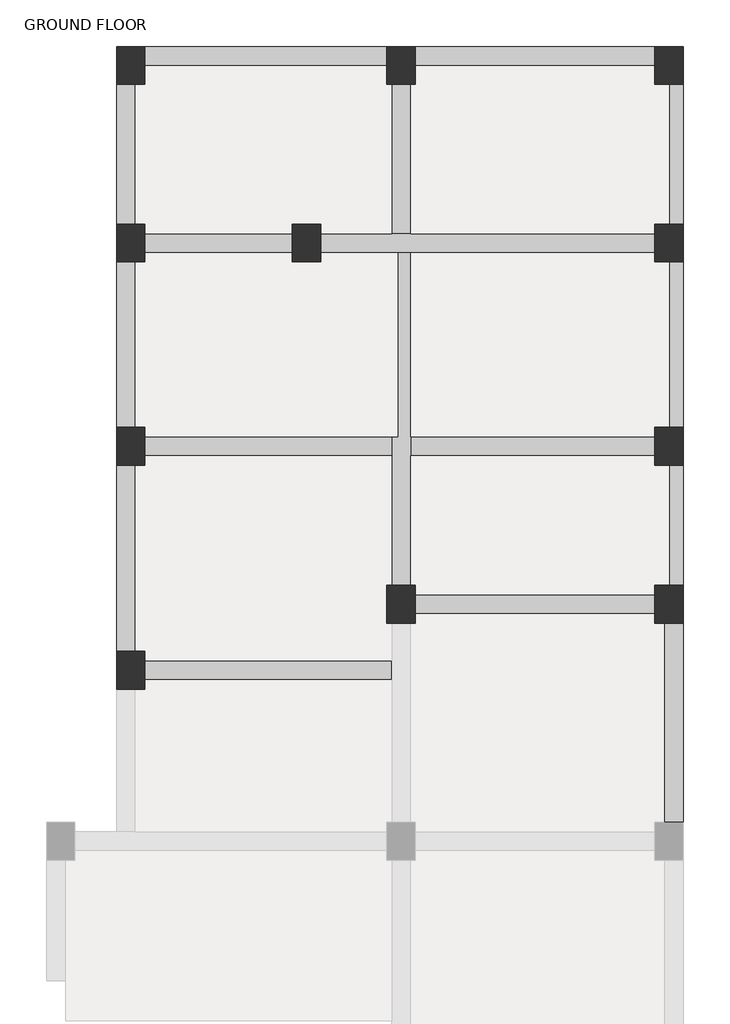
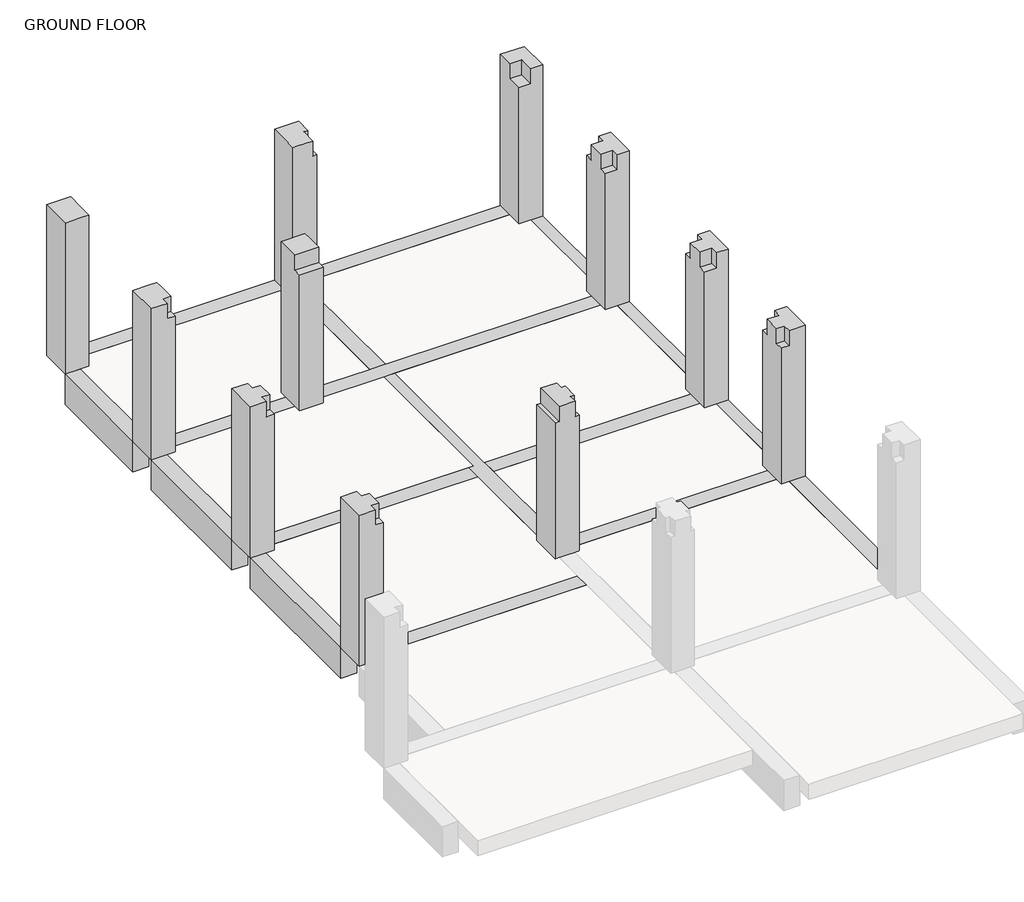
# One storey, part 2 of 2: 17 beams, 11 columns.
"""IFC4 building model written with IfcOpenShell, lengths in millimetres."""

from ifc_helpers import new_model, si_unit, frame, origin, place, context, project, spatial, polyline, outline, extrude, faceted_brep, element, save

model = new_model("IFC4")

# Units and contexts
model_context = context("Model", 3, world=origin())
ifc_project = project(units=[si_unit("LENGTHUNIT", "METRE", prefix="MILLI")], contexts=[model_context])

# Site, building, storey
site = spatial("IfcSite", under=ifc_project)
building = spatial("IfcBuilding", under=site)
storey = spatial("IfcBuildingStorey", under=building, Name="GROUND FLOOR", Elevation=0.0)

# Beams
placement = place(None, origin())
element("IfcBeam", 1, ObjectType="M_Concrete-Rectangular Beam : 300 x 600mm", at=placement, inside=storey, context=model_context, shape_type="Brep", body=[
    faceted_brep([(-2096.635935, 10150.0657956, 0.0), (-2096.635935, 10450.0657956, 0.0), (-5925.9642664, 10450.0657956, 0.0), (-5925.9642664, 10150.0657956, 0.0), (-2096.635935, 10150.0657956, -600.0), (-2096.635935, 10150.0657956, -300.0), (-5925.9642664, 10150.0657956, -300.0), (-5925.9642664, 10150.0657956, -600.0), (-2096.635935, 10450.0657956, -600.0), (-5925.9642664, 10450.0657956, -600.0)], [[[0, 1, 2, 3]], [[4, 5, 0, 3, 6, 7]], [[8, 4, 7, 9]], [[1, 8, 9, 2]], [[2, 9, 7, 6, 3]], [[1, 0, 5, 4, 8]]]),
])
element("IfcBeam", 2, ObjectType="M_Concrete-Rectangular Beam : 300 x 600mm", at=placement, inside=storey, context=model_context, shape_type="SweptSolid", body=[
    extrude(outline(polyline([(2143.5134108, 10450.0657956), (2143.5134108, 10150.0657956), (-1646.635935, 10150.0657956), (-1646.635935, 10450.0657956), (2143.5134108, 10450.0657956)])), frame((0.0, 0.0, -600.0), z_axis=(0.0, 0.0, 1.0), x_axis=(1.0, 0.0, 0.0)), (0.0, 0.0, 1.0), 600.0),
])
element("IfcBeam", 3, ObjectType="M_Concrete-Rectangular Beam : 300 x 600mm", at=placement, inside=storey, context=model_context, shape_type="Brep", body=[
    faceted_brep([(-6375.9642664, 7641.506653, 0.0), (-6075.9642664, 7641.506653, 0.0), (-6075.9642664, 9850.0657956, 0.0), (-6375.9642664, 9850.0657956, 0.0), (-6375.9642664, 7641.506653, -600.0), (-6375.9642664, 9850.0657956, -600.0), (-6075.9642664, 7641.506653, -600.0), (-6075.9642664, 9850.0657956, -600.0), (-6075.9642664, 7641.506653, -300.0), (-6075.9642664, 9850.0657956, -300.0)], [[[0, 1, 2, 3]], [[4, 0, 3, 5]], [[6, 4, 5, 7]], [[1, 8, 6, 7, 9, 2]], [[2, 9, 7, 5, 3]], [[1, 0, 4, 6, 8]]]),
])
element("IfcBeam", 4, ObjectType="M_Concrete-Rectangular Beam : 300 x 600mm", at=placement, inside=storey, context=model_context, shape_type="SweptSolid", body=[
    extrude(outline(polyline([(-6075.9642664, 4424.5351605), (-6375.9642664, 4424.5351605), (-6375.9642664, 7041.506653), (-6075.9642664, 7041.506653), (-6075.9642664, 4424.5351605)])), frame((0.0, 0.0, -600.0), z_axis=(0.0, 0.0, 1.0), x_axis=(1.0, 0.0, 0.0)), (0.0, 0.0, 1.0), 600.0),
])
element("IfcBeam", 5, ObjectType="M_Concrete-Rectangular Beam : 300 x 600mm", at=placement, inside=storey, context=model_context, shape_type="SweptSolid", body=[
    extrude(outline(polyline([(-6075.9642664, 881.5941646), (-6375.9642664, 881.5941646), (-6375.9642664, 3824.5351605), (-6075.9642664, 3824.5351605), (-6075.9642664, 881.5941646)])), frame((0.0, 0.0, -600.0), z_axis=(0.0, 0.0, 1.0), x_axis=(1.0, 0.0, 0.0)), (0.0, 0.0, 1.0), 600.0),
])
element("IfcBeam", 6, ObjectType="M_Concrete-Rectangular Beam : 300 x 600mm", at=placement, inside=storey, context=model_context, shape_type="SweptSolid", body=[
    extrude(outline(polyline([(2293.5134108, 1328.1057379), (2593.5134108, 1328.1057379), (2593.5134108, -1823.3693625), (2293.5134108, -1823.3693625), (2293.5134108, 1328.1057379)])), frame((0.0, 0.0, -600.0), z_axis=(0.0, 0.0, 1.0), x_axis=(1.0, 0.0, 0.0)), (0.0, 0.0, 1.0), 600.0),
])
element("IfcBeam", 7, ObjectType="M_Concrete-Rectangular Beam : 300 x 600mm", at=placement, inside=storey, context=model_context, shape_type="SweptSolid", body=[
    extrude(outline(polyline([(-600.0, 2293.5134108), (-600.0, 2593.5134108), (0.0, 2593.5134108), (0.0, 2368.5134108), (-300.0, 2368.5134108), (-300.0, 2293.5134108), (-600.0, 2293.5134108)])), frame((0.0, 1928.1057379, 0.0), z_axis=(0.0, 1.0, 0.0), x_axis=(0.0, 0.0, 1.0)), (0.0, 0.0, 1.0), 1896.4294226),
])
element("IfcBeam", 8, ObjectType="M_Concrete-Rectangular Beam : 300 x 600mm", at=placement, inside=storey, context=model_context, shape_type="SweptSolid", body=[
    extrude(outline(polyline([(-600.0, 2293.5134108), (-600.0, 2593.5134108), (0.0, 2593.5134108), (0.0, 2368.5134108), (-300.0, 2368.5134108), (-300.0, 2293.5134108), (-600.0, 2293.5134108)])), frame((0.0, 4424.5351605, 0.0), z_axis=(0.0, 1.0, 0.0), x_axis=(0.0, 0.0, 1.0)), (0.0, 0.0, 1.0), 2616.9714925),
])
element("IfcBeam", 9, ObjectType="M_Concrete-Rectangular Beam : 300 x 600mm", at=placement, inside=storey, context=model_context, shape_type="SweptSolid", body=[
    extrude(outline(polyline([(-600.0, 2293.5134108), (-600.0, 2593.5134108), (0.0, 2593.5134108), (0.0, 2368.5134108), (-300.0, 2368.5134108), (-300.0, 2293.5134108), (-600.0, 2293.5134108)])), frame((0.0, 7641.506653, 0.0), z_axis=(0.0, 1.0, 0.0), x_axis=(0.0, 0.0, 1.0)), (0.0, 0.0, 1.0), 2208.5591426),
])
element("IfcBeam", 10, ObjectType="M_Concrete-Rectangular Beam : 300 x 600mm", at=placement, inside=storey, context=model_context, shape_type="Brep", body=[
    faceted_brep([(-3596.635935, 7191.506653, 0.0), (-3596.635935, 7491.506653, 0.0), (-5925.9642664, 7491.506653, 0.0), (-5925.9642664, 7191.506653, 0.0), (-3596.635935, 7191.506653, -600.0), (-5925.9642664, 7191.506653, -600.0), (-3596.635935, 7491.506653, -600.0), (-5925.9642664, 7491.506653, -600.0), (-3596.635935, 7491.506653, -300.0), (-5925.9642664, 7491.506653, -300.0)], [[[0, 1, 2, 3]], [[4, 0, 3, 5]], [[6, 4, 5, 7]], [[1, 8, 6, 7, 9, 2]], [[2, 9, 7, 5, 3]], [[1, 0, 4, 6, 8]]]),
])
element("IfcBeam", 11, ObjectType="M_Concrete-Rectangular Beam : 300 x 600mm", at=placement, inside=storey, context=model_context, shape_type="Brep", body=[
    faceted_brep([(-3146.635935, 7491.506653, 0.0), (-3146.635935, 7191.506653, 0.0), (-1928.7254278, 7191.506653, 0.0), (-1721.635935, 7191.506653, 0.0), (2143.5134108, 7191.506653, 0.0), (2143.5134108, 7491.506653, 0.0), (-1721.635935, 7491.506653, 0.0), (-2021.635935, 7491.506653, 0.0), (-3146.635935, 7491.506653, -600.0), (-3146.635935, 7491.506653, -300.0), (2143.5134108, 7491.506653, -600.0), (-1721.635935, 7491.506653, -600.0), (-2021.635935, 7491.506653, -600.0), (-3146.635935, 7191.506653, -600.0), (2143.5134108, 7191.506653, -600.0), (-1721.635935, 7191.506653, -600.0), (-2021.635935, 7191.506653, -600.0)], [[[0, 1, 2, 3, 4, 5, 6, 7]], [[8, 9, 0, 7, 6, 5, 10, 11, 12]], [[13, 8, 12, 11, 10, 14, 15, 16]], [[1, 13, 16, 15, 14, 4, 3, 2]], [[1, 0, 9, 8, 13]], [[4, 14, 10, 5]]]),
])
element("IfcBeam", 12, ObjectType="M_Concrete-Rectangular Beam : 300 x 600mm", at=placement, inside=storey, context=model_context, shape_type="SweptSolid", body=[
    extrude(outline(polyline([(-1646.635935, 1478.1057379), (-1646.635935, 1778.1057379), (2143.5134108, 1778.1057379), (2143.5134108, 1478.1057379), (-1646.635935, 1478.1057379)])), frame((0.0, 0.0, -600.0), z_axis=(0.0, 0.0, 1.0), x_axis=(1.0, 0.0, 0.0)), (0.0, 0.0, 1.0), 600.0),
])
element("IfcBeam", 13, ObjectType="M_Concrete-Rectangular Beam : 300 x 600mm", at=placement, inside=storey, context=model_context, shape_type="Brep", body=[
    faceted_brep([(-1721.635935, 9850.0657956, 0.0), (-2021.635935, 9850.0657956, 0.0), (-2021.635935, 7491.506653, 0.0), (-1721.635935, 7491.506653, 0.0), (-2021.635935, 9850.0657956, -300.0), (-2021.635935, 9850.0657956, -600.0), (-2021.635935, 7491.506653, -600.0), (-2021.635935, 7491.506653, -300.0), (-1721.635935, 9850.0657956, -600.0), (-1721.635935, 7491.506653, -600.0), (-1721.635935, 7491.506653, -300.0)], [[[0, 1, 2, 3]], [[1, 4, 5, 6, 7, 2]], [[5, 8, 9, 6]], [[8, 0, 3, 10, 9]], [[0, 8, 5, 4, 1]], [[3, 2, 7, 6, 9, 10]]]),
])
element("IfcBeam", 14, ObjectType="M_Concrete-Rectangular Beam : 300 x 600mm", at=placement, inside=storey, context=model_context, shape_type="Brep", body=[
    faceted_brep([(-2021.635935, 1928.1057379, 0.0), (-1721.635935, 1928.1057379, 0.0), (-1721.635935, 3974.5351605, 0.0), (-1721.635935, 4274.5351605, 0.0), (-1721.635935, 7191.506653, 0.0), (-1928.7254278, 7191.506653, 0.0), (-1928.7254278, 4274.5351605, 0.0), (-2021.635935, 4274.5351605, 0.0), (-2021.635935, 3974.5351605, 0.0), (-1721.635935, 1928.1057379, -600.0), (-1721.635935, 3974.5351605, -600.0), (-1721.635935, 4274.5351605, -600.0), (-1721.635935, 7191.506653, -600.0), (-1721.635935, 7191.506653, -300.0), (-2021.635935, 1928.1057379, -600.0), (-2021.635935, 3974.5351605, -600.0), (-2021.635935, 4274.5351605, -600.0), (-2021.635935, 7191.506653, -600.0), (-2021.635935, 4274.5351605, -300.0), (-2021.635935, 7191.506653, -300.0), (-1928.7254278, 7191.506653, -300.0), (-1928.7254278, 4274.5351605, -300.0)], [[[0, 1, 2, 3, 4, 5, 6, 7, 8]], [[1, 9, 10, 11, 12, 13, 4, 3, 2]], [[9, 14, 15, 16, 17, 12, 11, 10]], [[14, 0, 8, 7, 18, 19, 17, 16, 15]], [[0, 14, 9, 1]], [[4, 13, 12, 17, 19, 20, 5]], [[21, 20, 19, 18]], [[20, 21, 6, 5]], [[6, 21, 18, 7]]]),
])
element("IfcBeam", 15, ObjectType="M_Concrete-Rectangular Beam : 300 x 600mm", at=placement, inside=storey, context=model_context, shape_type="Brep", body=[
    faceted_brep([(-5925.9642664, 731.5941646, 0.0), (-5925.9642664, 431.5941646, 0.0), (-2021.635935, 431.5941646, 0.0), (-2021.635935, 731.5941646, 0.0), (-5925.9642664, 431.5941646, -600.0), (-2021.635935, 431.5941646, -600.0), (-2021.635935, 431.5941646, -300.0), (-5925.9642664, 731.5941646, -600.0), (-2021.635935, 731.5941646, -600.0), (-2021.635935, 731.5941646, -300.0)], [[[0, 1, 2, 3]], [[1, 4, 5, 6, 2]], [[4, 7, 8, 5]], [[7, 0, 3, 9, 8]], [[0, 7, 4, 1]], [[3, 2, 6, 5, 8, 9]]]),
])
element("IfcBeam", 16, ObjectType="M_Concrete-Rectangular Beam : 300 x 600mm", at=placement, inside=storey, context=model_context, shape_type="Brep", body=[
    faceted_brep([(-5925.9642664, 4274.5351605, 0.0), (-5925.9642664, 3974.5351605, 0.0), (-2021.635935, 3974.5351605, 0.0), (-2021.635935, 4274.5351605, 0.0), (-5925.9642664, 3974.5351605, -600.0), (-2021.635935, 3974.5351605, -600.0), (-2021.635935, 3974.5351605, -300.0), (-5925.9642664, 4274.5351605, -600.0), (-2021.635935, 4274.5351605, -600.0), (-2021.635935, 4274.5351605, -300.0)], [[[0, 1, 2, 3]], [[1, 4, 5, 6, 2]], [[4, 7, 8, 5]], [[7, 0, 3, 9, 8]], [[0, 7, 4, 1]], [[3, 2, 6, 5, 8, 9]]]),
])
element("IfcBeam", 17, ObjectType="M_Concrete-Rectangular Beam : 300 x 600mm", at=placement, inside=storey, context=model_context, shape_type="Brep", body=[
    faceted_brep([(2143.5134108, 3974.5351605, 0.0), (2143.5134108, 4274.5351605, 0.0), (-1721.635935, 4274.5351605, 0.0), (-1721.635935, 3974.5351605, 0.0), (2143.5134108, 4274.5351605, -600.0), (-1721.635935, 4274.5351605, -600.0), (-1721.635935, 4274.5351605, -300.0), (2143.5134108, 3974.5351605, -600.0), (-1721.635935, 3974.5351605, -600.0), (-1721.635935, 3974.5351605, -300.0)], [[[0, 1, 2, 3]], [[1, 4, 5, 6, 2]], [[4, 7, 8, 5]], [[7, 0, 3, 9, 8]], [[0, 7, 4, 1]], [[3, 2, 6, 5, 8, 9]]]),
])

# Columns
element("IfcColumn", 18, ObjectType="M_Concrete-Rectangular-Column : 450 x 600mm", at=placement, inside=storey, context=model_context, shape_type="Brep", body=[
    faceted_brep([(-5925.9642664, 10450.0657956, 0.0), (-5925.9642664, 9850.0657956, 0.0), (-6375.9642664, 9850.0657956, 0.0), (-6375.9642664, 10450.0657956, 0.0), (-5925.9642664, 10450.0657956, 3000.0), (-5925.9642664, 10150.0657956, 3000.0), (-5925.9642664, 9850.0657956, 3000.0), (-5925.9642664, 9850.0657956, 2700.0), (-6075.9642664, 9850.0657956, 3000.0), (-6375.9642664, 9850.0657956, 3000.0), (-6375.9642664, 10450.0657956, 3000.0)], [[[0, 1, 2, 3]], [[1, 0, 4, 5, 6, 7]], [[2, 1, 7, 6, 8, 9]], [[3, 2, 9, 10]], [[0, 3, 10, 4]], [[10, 9, 8, 6, 5, 4]]]),
])
element("IfcColumn", 19, ObjectType="M_Concrete-Rectangular-Column : 450 x 600mm", at=placement, inside=storey, context=model_context, shape_type="Brep", body=[
    faceted_brep([(-5925.9642664, 7641.506653, 0.0), (-5925.9642664, 7041.506653, 0.0), (-6375.9642664, 7041.506653, 0.0), (-6375.9642664, 7641.506653, 0.0), (-5925.9642664, 7641.506653, 2700.0), (-5925.9642664, 7641.506653, 3000.0), (-5925.9642664, 7491.506653, 3000.0), (-5925.9642664, 7191.506653, 3000.0), (-5925.9642664, 7191.506653, 2700.0), (-5925.9642664, 7041.506653, 2700.0), (-6075.9642664, 7041.506653, 2700.0), (-6075.9642664, 7041.506653, 3000.0), (-6375.9642664, 7041.506653, 3000.0), (-6375.9642664, 7641.506653, 3000.0), (-6075.9642664, 7641.506653, 3000.0), (-6075.9642664, 7191.506653, 3000.0), (-6075.9642664, 7191.506653, 2700.0)], [[[0, 1, 2, 3]], [[1, 0, 4, 5, 6, 7, 8, 9]], [[2, 1, 9, 10, 11, 12]], [[3, 2, 12, 13]], [[0, 3, 13, 14, 5, 4]], [[13, 12, 11, 15, 7, 6, 5, 14]], [[16, 10, 9, 8]], [[15, 16, 8, 7]], [[16, 15, 11, 10]]]),
])
element("IfcColumn", 20, ObjectType="M_Concrete-Rectangular-Column : 450 x 600mm", at=placement, inside=storey, context=model_context, shape_type="Brep", body=[
    faceted_brep([(-5925.9642664, 4424.5351605, 0.0), (-5925.9642664, 3824.5351605, 0.0), (-6375.9642664, 3824.5351605, 0.0), (-6375.9642664, 4424.5351605, 0.0), (-5925.9642664, 4424.5351605, 2700.0), (-5925.9642664, 4274.5351605, 2700.0), (-5925.9642664, 4274.5351605, 3000.0), (-5925.9642664, 3974.5351605, 3000.0), (-5925.9642664, 3974.5351605, 2700.0), (-5925.9642664, 3824.5351605, 2700.0), (-6075.9642664, 3824.5351605, 2700.0), (-6075.9642664, 3824.5351605, 3000.0), (-6375.9642664, 3824.5351605, 3000.0), (-6375.9642664, 4424.5351605, 3000.0), (-6075.9642664, 4424.5351605, 3000.0), (-6075.9642664, 4424.5351605, 2700.0), (-6075.9642664, 3974.5351605, 3000.0), (-6075.9642664, 4274.5351605, 3000.0), (-6075.9642664, 4274.5351605, 2700.0), (-6075.9642664, 3974.5351605, 2700.0)], [[[0, 1, 2, 3]], [[1, 0, 4, 5, 6, 7, 8, 9]], [[2, 1, 9, 10, 11, 12]], [[3, 2, 12, 13]], [[0, 3, 13, 14, 15, 4]], [[13, 12, 11, 16, 7, 6, 17, 14]], [[15, 18, 5, 4]], [[18, 17, 6, 5]], [[17, 18, 15, 14]], [[19, 10, 9, 8]], [[16, 19, 8, 7]], [[19, 16, 11, 10]]]),
])
element("IfcColumn", 21, ObjectType="M_Concrete-Rectangular-Column : 450 x 600mm", at=placement, inside=storey, context=model_context, shape_type="Brep", body=[
    faceted_brep([(-5925.9642664, 881.5941646, 0.0), (-5925.9642664, 281.5941646, 0.0), (-6375.9642664, 281.5941646, 0.0), (-6375.9642664, 881.5941646, 0.0), (-5925.9642664, 881.5941646, 2700.0), (-5925.9642664, 731.5941646, 2700.0), (-5925.9642664, 731.5941646, 3000.0), (-5925.9642664, 431.5941646, 3000.0), (-5925.9642664, 431.5941646, 2700.0), (-5925.9642664, 281.5941646, 2700.0), (-6075.9642664, 281.5941646, 2700.0), (-6075.9642664, 281.5941646, 3000.0), (-6375.9642664, 281.5941646, 3000.0), (-6375.9642664, 881.5941646, 3000.0), (-6075.9642664, 881.5941646, 3000.0), (-6075.9642664, 881.5941646, 2700.0), (-6075.9642664, 431.5941646, 3000.0), (-6075.9642664, 731.5941646, 3000.0), (-6075.9642664, 731.5941646, 2700.0), (-6075.9642664, 431.5941646, 2700.0)], [[[0, 1, 2, 3]], [[1, 0, 4, 5, 6, 7, 8, 9]], [[2, 1, 9, 10, 11, 12]], [[3, 2, 12, 13]], [[0, 3, 13, 14, 15, 4]], [[13, 12, 11, 16, 7, 6, 17, 14]], [[15, 18, 5, 4]], [[18, 17, 6, 5]], [[17, 18, 15, 14]], [[19, 10, 9, 8]], [[19, 16, 11, 10]], [[16, 19, 8, 7]]]),
])
element("IfcColumn", 22, ObjectType="M_Concrete-Rectangular-Column : 450 x 600mm", at=placement, inside=storey, context=model_context, shape_type="Brep", body=[
    faceted_brep([(-3146.635935, 7641.506653, 0.0), (-3146.635935, 7041.506653, 0.0), (-3596.635935, 7041.506653, 0.0), (-3596.635935, 7641.506653, 0.0), (-3146.635935, 7641.506653, 2700.0), (-3146.635935, 7641.506653, 3000.0), (-3146.635935, 7491.506653, 3000.0), (-3146.635935, 7191.506653, 3000.0), (-3146.635935, 7191.506653, 2700.0), (-3146.635935, 7041.506653, 2700.0), (-3596.635935, 7041.506653, 2700.0), (-3596.635935, 7191.506653, 2700.0), (-3596.635935, 7191.506653, 3000.0), (-3596.635935, 7491.506653, 3000.0), (-3596.635935, 7641.506653, 3000.0), (-3596.635935, 7641.506653, 2700.0)], [[[0, 1, 2, 3]], [[1, 0, 4, 5, 6, 7, 8, 9]], [[2, 1, 9, 10]], [[3, 2, 10, 11, 12, 13, 14, 15]], [[0, 3, 15, 14, 5, 4]], [[5, 14, 13, 12, 7, 6]], [[8, 11, 10, 9]], [[11, 8, 7, 12]]]),
])
element("IfcColumn", 23, ObjectType="M_Concrete-Rectangular-Column : 450 x 600mm", at=placement, inside=storey, context=model_context, shape_type="Brep", body=[
    faceted_brep([(-1646.635935, 10450.0657956, 0.0), (-1646.635935, 9850.0657956, 0.0), (-2096.635935, 9850.0657956, 0.0), (-2096.635935, 10450.0657956, 0.0), (-1646.635935, 10450.0657956, 3000.0), (-1646.635935, 10150.0657956, 3000.0), (-1646.635935, 10150.0657956, 2700.0), (-1646.635935, 9850.0657956, 2700.0), (-1721.635935, 9850.0657956, 2700.0), (-1721.635935, 9850.0657956, 3000.0), (-2021.635935, 9850.0657956, 3000.0), (-2096.635935, 9850.0657956, 3000.0), (-2096.635935, 9850.0657956, 2700.0), (-2096.635935, 10150.0657956, 3000.0), (-2096.635935, 10450.0657956, 3000.0), (-1721.635935, 10150.0657956, 3000.0), (-1721.635935, 10150.0657956, 2700.0)], [[[0, 1, 2, 3]], [[1, 0, 4, 5, 6, 7]], [[2, 1, 7, 8, 9, 10, 11, 12]], [[3, 2, 12, 11, 13, 14]], [[0, 3, 14, 4]], [[4, 14, 13, 11, 10, 9, 15, 5]], [[16, 8, 7, 6]], [[15, 16, 6, 5]], [[16, 15, 9, 8]]]),
])
element("IfcColumn", 24, ObjectType="M_Concrete-Rectangular-Column : 450 x 600mm", at=placement, inside=storey, context=model_context, shape_type="Brep", body=[
    faceted_brep([(-1646.635935, 1928.1057379, 0.0), (-1646.635935, 1328.1057379, 0.0), (-2096.635935, 1328.1057379, 0.0), (-2096.635935, 1928.1057379, 0.0), (-1646.635935, 1928.1057379, 2700.0), (-1646.635935, 1778.1057379, 2700.0), (-1646.635935, 1778.1057379, 3000.0), (-1646.635935, 1478.1057379, 3000.0), (-1646.635935, 1478.1057379, 2700.0), (-1646.635935, 1328.1057379, 2700.0), (-1721.635935, 1328.1057379, 2700.0), (-1721.635935, 1328.1057379, 3000.0), (-2021.635935, 1328.1057379, 3000.0), (-2021.635935, 1328.1057379, 2700.0), (-2096.635935, 1328.1057379, 2700.0), (-2096.635935, 1928.1057379, 2700.0), (-2021.635935, 1928.1057379, 2700.0), (-2021.635935, 1928.1057379, 3000.0), (-1721.635935, 1928.1057379, 3000.0), (-1721.635935, 1928.1057379, 2700.0), (-1721.635935, 1778.1057379, 3000.0), (-1721.635935, 1478.1057379, 3000.0), (-1721.635935, 1778.1057379, 2700.0), (-1721.635935, 1478.1057379, 2700.0)], [[[0, 1, 2, 3]], [[1, 0, 4, 5, 6, 7, 8, 9]], [[2, 1, 9, 10, 11, 12, 13, 14]], [[3, 2, 14, 15]], [[0, 3, 15, 16, 17, 18, 19, 4]], [[6, 20, 18, 17, 12, 11, 21, 7]], [[19, 22, 5, 4]], [[22, 20, 6, 5]], [[20, 22, 19, 18]], [[23, 10, 9, 8]], [[21, 23, 8, 7]], [[23, 21, 11, 10]], [[13, 16, 15, 14]], [[16, 13, 12, 17]]]),
])
element("IfcColumn", 25, ObjectType="M_Concrete-Rectangular-Column : 450 x 600mm", at=placement, inside=storey, context=model_context, shape_type="Brep", body=[
    faceted_brep([(2593.5134108, 10450.0657956, 0.0), (2593.5134108, 9850.0657956, 0.0), (2143.5134108, 9850.0657956, 0.0), (2143.5134108, 10450.0657956, 0.0), (2593.5134108, 10450.0657956, 3000.0), (2593.5134108, 9850.0657956, 3000.0), (2368.5134108, 9850.0657956, 3000.0), (2368.5134108, 9850.0657956, 2700.0), (2143.5134108, 9850.0657956, 2700.0), (2143.5134108, 10150.0657956, 2700.0), (2143.5134108, 10150.0657956, 3000.0), (2143.5134108, 10450.0657956, 3000.0), (2368.5134108, 10150.0657956, 3000.0), (2368.5134108, 10150.0657956, 2700.0)], [[[0, 1, 2, 3]], [[1, 0, 4, 5]], [[2, 1, 5, 6, 7, 8]], [[3, 2, 8, 9, 10, 11]], [[0, 3, 11, 4]], [[5, 4, 11, 10, 12, 6]], [[7, 13, 9, 8]], [[13, 12, 10, 9]], [[12, 13, 7, 6]]]),
])
element("IfcColumn", 26, ObjectType="M_Concrete-Rectangular-Column : 450 x 600mm", at=placement, inside=storey, context=model_context, shape_type="Brep", body=[
    faceted_brep([(2593.5134108, 7641.506653, 0.0), (2593.5134108, 7041.506653, 0.0), (2143.5134108, 7041.506653, 0.0), (2143.5134108, 7641.506653, 0.0), (2593.5134108, 7641.506653, 3000.0), (2593.5134108, 7041.506653, 3000.0), (2368.5134108, 7041.506653, 3000.0), (2368.5134108, 7041.506653, 2700.0), (2143.5134108, 7041.506653, 2700.0), (2143.5134108, 7191.506653, 2700.0), (2143.5134108, 7191.506653, 3000.0), (2143.5134108, 7491.506653, 3000.0), (2143.5134108, 7491.506653, 2700.0), (2143.5134108, 7641.506653, 2700.0), (2368.5134108, 7641.506653, 2700.0), (2368.5134108, 7641.506653, 3000.0), (2368.5134108, 7491.506653, 3000.0), (2368.5134108, 7191.506653, 3000.0), (2368.5134108, 7491.506653, 2700.0), (2368.5134108, 7191.506653, 2700.0)], [[[0, 1, 2, 3]], [[1, 0, 4, 5]], [[2, 1, 5, 6, 7, 8]], [[3, 2, 8, 9, 10, 11, 12, 13]], [[0, 3, 13, 14, 15, 4]], [[5, 4, 15, 16, 11, 10, 17, 6]], [[12, 18, 14, 13]], [[18, 16, 15, 14]], [[16, 18, 12, 11]], [[7, 19, 9, 8]], [[19, 17, 10, 9]], [[17, 19, 7, 6]]]),
])
element("IfcColumn", 27, ObjectType="M_Concrete-Rectangular-Column : 450 x 600mm", at=placement, inside=storey, context=model_context, shape_type="Brep", body=[
    faceted_brep([(2593.5134108, 4424.5351605, 0.0), (2593.5134108, 3824.5351605, 0.0), (2143.5134108, 3824.5351605, 0.0), (2143.5134108, 4424.5351605, 0.0), (2593.5134108, 4424.5351605, 3000.0), (2593.5134108, 3824.5351605, 3000.0), (2368.5134108, 3824.5351605, 3000.0), (2368.5134108, 3824.5351605, 2700.0), (2143.5134108, 3824.5351605, 2700.0), (2143.5134108, 3974.5351605, 2700.0), (2143.5134108, 3974.5351605, 3000.0), (2143.5134108, 4274.5351605, 3000.0), (2143.5134108, 4274.5351605, 2700.0), (2143.5134108, 4424.5351605, 2700.0), (2368.5134108, 4424.5351605, 2700.0), (2368.5134108, 4424.5351605, 3000.0), (2368.5134108, 4274.5351605, 3000.0), (2368.5134108, 3974.5351605, 3000.0), (2368.5134108, 4274.5351605, 2700.0), (2368.5134108, 3974.5351605, 2700.0)], [[[0, 1, 2, 3]], [[1, 0, 4, 5]], [[2, 1, 5, 6, 7, 8]], [[3, 2, 8, 9, 10, 11, 12, 13]], [[0, 3, 13, 14, 15, 4]], [[5, 4, 15, 16, 11, 10, 17, 6]], [[12, 18, 14, 13]], [[18, 16, 15, 14]], [[16, 18, 12, 11]], [[7, 19, 9, 8]], [[17, 19, 7, 6]], [[19, 17, 10, 9]]]),
])
element("IfcColumn", 28, ObjectType="M_Concrete-Rectangular-Column : 450 x 600mm", at=placement, inside=storey, context=model_context, shape_type="Brep", body=[
    faceted_brep([(2593.5134108, 1928.1057379, 0.0), (2593.5134108, 1328.1057379, 0.0), (2143.5134108, 1328.1057379, 0.0), (2143.5134108, 1928.1057379, 0.0), (2593.5134108, 1928.1057379, 3000.0), (2593.5134108, 1328.1057379, 3000.0), (2293.5134108, 1328.1057379, 3000.0), (2293.5134108, 1328.1057379, 2700.0), (2143.5134108, 1328.1057379, 2700.0), (2143.5134108, 1478.1057379, 2700.0), (2143.5134108, 1478.1057379, 3000.0), (2143.5134108, 1778.1057379, 3000.0), (2143.5134108, 1778.1057379, 2700.0), (2143.5134108, 1928.1057379, 2700.0), (2368.5134108, 1928.1057379, 2700.0), (2368.5134108, 1928.1057379, 3000.0), (2368.5134108, 1778.1057379, 3000.0), (2293.5134108, 1478.1057379, 3000.0), (2368.5134108, 1778.1057379, 2700.0), (2293.5134108, 1478.1057379, 2700.0)], [[[0, 1, 2, 3]], [[1, 0, 4, 5]], [[2, 1, 5, 6, 7, 8]], [[3, 2, 8, 9, 10, 11, 12, 13]], [[0, 3, 13, 14, 15, 4]], [[5, 4, 15, 16, 11, 10, 17, 6]], [[12, 18, 14, 13]], [[18, 16, 15, 14]], [[16, 18, 12, 11]], [[7, 19, 9, 8]], [[19, 17, 10, 9]], [[17, 19, 7, 6]]]),
])

save(model, "model.ifc")

# Revit data of these elements
# Type "M_Concrete-Rectangular Beam : 300 x 600mm"
#   Length [instance default] = 1524 mm
#   b = 300 mm
#   h = 600 mm
#   Structural Material [instance default] = Concrete, Cast-in-Place gray
#   Assembly Code = ""
# Type "M_Concrete-Rectangular-Column : 450 x 600mm"
#   b = 450 mm
#   h = 600 mm
#   Structural Material [instance default] = Concrete, Cast-in-Place gray
# Elements 1, 2, 3, 4, 5, 6, 7, 8, 9, 10, 11, 12, 13, 14, 15, 16, 17 (IfcBeam, "M_Concrete-Rectangular Beam : 300 x 600mm")
#   Structural Material = Concrete, Cast-in-Place gray
#   Phase Created = New Construction
#   Materials on its faces: "Concrete, Cast-in-Place gray"
# Elements 18, 19, 20, 21, 22, 23, 24, 25, 26, 27, 28 (IfcColumn, "M_Concrete-Rectangular-Column : 450 x 600mm")
#   Structural Material = Concrete, Cast-in-Place gray
#   Phase Created = New Construction
#   Materials on its faces: "Concrete, Cast-in-Place gray"
# Materials
#   "Concrete, Cast-in-Place gray": class "Concrete", colour RGB 192 192 192, transparency 0, Description = "Cast-in-place concrete", Cost = 0
